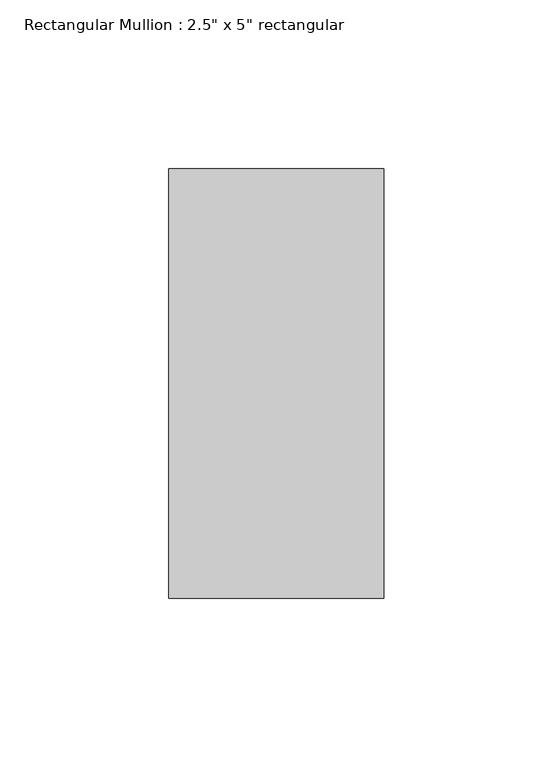
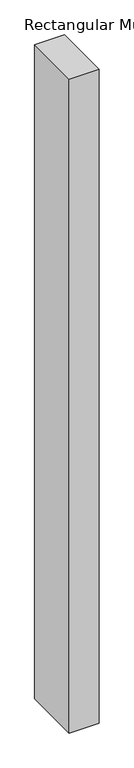
"""IFC4 building model written with IfcOpenShell, lengths in millimetres: member geometry."""

from ifc_helpers import new_model, si_unit, frame, origin, place, context, project, spatial, polyline, outline, extrude, source, transform, mapped, element, save


def member_c4e92d7b(model_context):
    return source(origin(), model_context, "Body", "SweptSolid", [
        extrude(outline(polyline([(0.0, 63.5), (0.0, -63.5), (-63.5, -63.5), (-63.5, 63.5), (0.0, 63.5)])), frame((0.0, 0.0, -1472.0504916), z_axis=(0.0, 0.0, 1.0), x_axis=(1.0, 0.0, 0.0)), (0.0, 0.0, 1.0), 1472.0504916),
    ])


if __name__ == "__main__":
    model = new_model("IFC4")
    model_context = context("Model", 3, world=origin())
    ifc_project = project(units=[si_unit("LENGTHUNIT", "METRE", prefix="MILLI")], contexts=[model_context])
    site = spatial("IfcSite", under=ifc_project)
    building = spatial("IfcBuilding", under=site)
    placement = place(None, origin())
    member_shape = member_c4e92d7b(model_context)
    element("IfcMember", 1, ObjectType="Rectangular Mullion : 2.5\" x 5\" rectangular", at=placement, inside=building, context=model_context, shape_type="MappedRepresentation", body=[
        mapped(member_shape, transform((0.0, 0.0, 0.0), x_axis=(1.0, 0.0, 0.0), y_axis=(0.0, 1.0, 0.0), z_axis=(0.0, 0.0, 1.0))),
    ])
    save(model, "model.ifc")

# Revit data of these elements
# Type "Rectangular Mullion : 2.5\" x 5\" rectangular"
#   built-in parameter 1007304 = 0.416667 (stored number, unit not read)
#   built-in parameter 1007301 = 0.104167 (stored number, unit not read)
#   built-in parameter 1007300 = 0.104167 (stored number, unit not read)
# Element 1 (IfcMember, "Rectangular Mullion : 2.5\" x 5\" rectangular")
#   Materials on its faces: "Aluminum"
# Materials
#   "Aluminum": class "Metal", colour RGB 247 247 247, transparency 0, Description = "Aluminum 6061", Cost = 0
